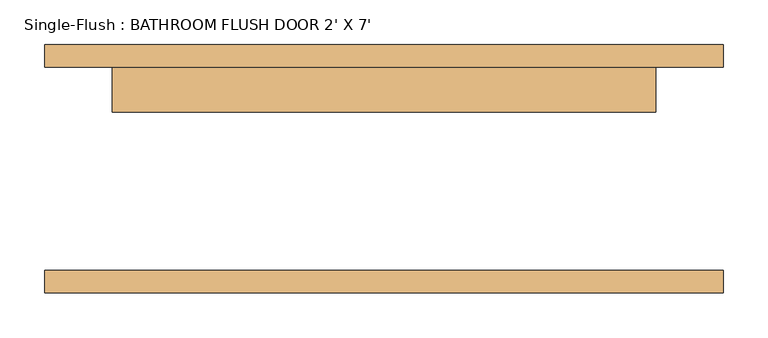
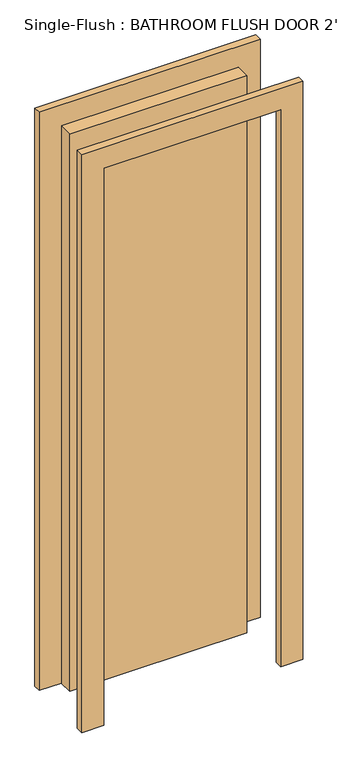
"""IFC4 building model written with IfcOpenShell, lengths in millimetres: door geometry, Single-Flush : BATHROOM FLUSH DOOR 2' X 7'."""

from ifc_helpers import new_model, si_unit, frame, origin, origin_with_axes, place, context, project, spatial, polyline, outline, extrude, source, transform, mapped, element, save


def single_flush_bathroom_flush_door_2_x_7_88cc3d71(model_context):
    return source(origin(), model_context, "Body", "SweptSolid", [
        extrude(outline(polyline([(2108.2, -381.0), (0.0, -381.0), (0.0, -304.8), (2032.0, -304.8), (2032.0, 304.8), (0.0, 304.8), (0.0, 381.0), (2108.2, 381.0), (2108.2, -381.0)])), frame((0.0, 114.3, 0.0), z_axis=(0.0, 1.0, 0.0), x_axis=(0.0, 0.0, 1.0)), (0.0, 0.0, 1.0), 25.4),
        extrude(outline(polyline([(2108.2, 381.0), (2108.2, -381.0), (0.0, -381.0), (0.0, -304.8), (2032.0, -304.8), (2032.0, 304.8), (0.0, 304.8), (0.0, 381.0), (2108.2, 381.0)])), frame((0.0, -139.7, 0.0), z_axis=(0.0, 1.0, 0.0), x_axis=(0.0, 0.0, 1.0)), (0.0, 0.0, 1.0), 25.4),
        extrude(outline(polyline([(304.8, 63.5), (-304.8, 63.5), (-304.8, 114.3), (304.8, 114.3), (304.8, 63.5)])), origin_with_axes(), (0.0, 0.0, 1.0), 2032.0),
    ])


if __name__ == "__main__":
    model = new_model("IFC4")
    model_context = context("Model", 3, world=origin())
    ifc_project = project(units=[si_unit("LENGTHUNIT", "METRE", prefix="MILLI")], contexts=[model_context])
    site = spatial("IfcSite", under=ifc_project)
    building = spatial("IfcBuilding", under=site)
    placement = place(None, origin())
    single_flush_bathroom_flush_door_2_x_7_shape = single_flush_bathroom_flush_door_2_x_7_88cc3d71(model_context)
    element("IfcDoor", 1, ObjectType="Single-Flush : BATHROOM FLUSH DOOR 2' X 7'", at=placement, inside=building, context=model_context, shape_type="MappedRepresentation", body=[
        mapped(single_flush_bathroom_flush_door_2_x_7_shape, transform((0.0, 0.0, 0.0), x_axis=(1.0, 0.0, 0.0), y_axis=(0.0, 1.0, 0.0), z_axis=(0.0, 0.0, 1.0))),
    ])
    save(model, "model.ifc")

# Revit data of these elements
# Type "Single-Flush : BATHROOM FLUSH DOOR 2' X 7'"
#   Type Mark = "8"
#   Construction Type Id = "MDOOR"
#   Assembly Code = "C1020"
#   Analytic Construction = "Metal"
#   Thickness = 0' - 2"
#   Heat Transfer Coefficient (U) = 0.651978 BTU/(h·ft²·°F)
#   Height = 6' - 8"
#   Trim Projection Ext = 0' - 1"
#   Trim Projection Int = 0' - 1"
#   Trim Width = 0' - 3"
#   Width = 2' - 0"
#   Define Thermal Properties by = 1
#   Door Material = Door - Panel
#   Frame Material = Door - Frame
#   Visual Light Transmittance = 0
#   Solar Heat Gain Coefficient = 0
#   Function = (empty or 0)
#   Wall Closure = (empty or 0)
# Element 1 (IfcDoor, "Single-Flush : BATHROOM FLUSH DOOR 2' X 7'")
#   Materials on its faces: "Door - Frame", "Door - Panel"
# Materials
#   "Door - Panel": class "Wood", colour RGB 210 159 95, transparency 0, Cost = 0
#   "Door - Frame": colour RGB 118 70 51, transparency 0, Cost = 0
